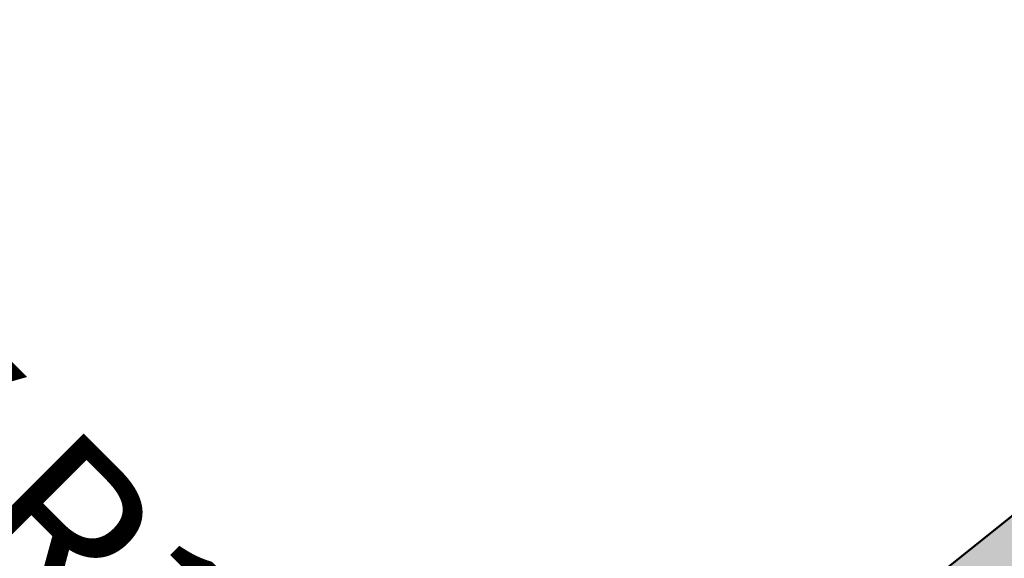
# Model space of a CAD drawing. Units: millimetres. Extents: x 0 to 2267, y 0 to 1823.
# Tile 19 of 256: x 1506 to 1548, y 1139 to 1162. Entities that reach past the tile are written whole.
import ezdxf

# ---------------------------------------------------------------- set-up
doc = ezdxf.new("R2010")
doc.units = ezdxf.units.MM
doc.header["$MEASUREMENT"] = 0
for name, color, linetype, lineweight in [('M-DIMS', 2, 'Continuous', 25), ('M-HATC', 252, 'Continuous', 18), ('M-OUTL', 7, 'Continuous', 50)]:
    doc.layers.add(name, color=color, linetype=linetype, lineweight=lineweight)
doc.styles.get("Standard").update_dxf_attribs({"font": 'arial.ttf'})
doc.dimstyles.get("Standard").update_dxf_attribs({"dimtxt": 7, "dimasz": 4, "dimexe": 0.18, "dimexo": 0.0625, "dimgap": 0.09, "dimtad": 0, "dimdec": 0, "dimzin": 0, "dimdsep": 46, "dimtxsty": 'Standard', "dimcen": 0.09, "dimadec": 0, "dimazin": 0, "dimtfac": 1, "dimtdec": 0, "dimtofl": 0, "dimtmove": 0, "dimatfit": 3, "dimfxl": 1, "dimtolj": 1, "dimtzin": 0, "dimarcsym": 0})

# ---------------------------------------------------------------- blocks, each defined once
blk = doc.blocks.new('*D28')
at = {"layer": 'Defpoints', "color": 0, "transparency": 16777216}
for p in [(1523.858, 1124.488), (1530.929, 1117.417)]:
    blk.add_point(p, dxfattribs=at)
at = {"layer": 'M-DIMS', "color": 0, "lineweight": -2, "transparency": 16777216}
for p, q in [((1518.201, 1130.145), (1521.029, 1127.317)), ((1530.929, 1117.327), (1530.929, 1117.507)), ((1530.839, 1117.417), (1531.019, 1117.417))]:
    blk.add_line(p, q, dxfattribs=at)
at = {"layer": 'M-DIMS', "color": 0, "transparency": 16777216}
blk.add_solid([(1521.501, 1127.788), (1520.558, 1126.845), (1523.858, 1124.488)], dxfattribs=at)
at = {"layer": 'M-DIMS', "color": 0, "transparency": 16777216, "insert": (1504.949, 1143.397), "char_height": 7, "attachment_point": 5, "rotation": 314.9998}
blk.add_mtext('\\A1;27X R10', dxfattribs=at)

msp = doc.modelspace()

# ---------------------------------------------------------------- hatches: boundary and pattern name
at = {"layer": 'M-HATC'}
h = msp.add_hatch(color=256, dxfattribs=at)
h.dxf.hatch_style = 1
h.paths.add_polyline_path([(2055.771, 1603.062), (1381.087, 1603.062), (1381.087, 1598.062), (2055.771, 1598.062)])
h.paths.add_polyline_path([(2055.771, 1598.062), (1381.087, 1598.062), (1381.087, 1593.062), (2055.771, 1593.062)])
h.paths.add_polyline_path([(2051.307, 1536.761), (1385.55, 1536.761), (1385.55, 1526.761), (1387.55, 1526.761), (1388.537, 1525.053), (1385.332, 1521.233), (1385.332, 1521.223), (2050.254, 1522.749), (2048.321, 1525.053), (2049.307, 1526.761), (2051.307, 1526.761)])
edge = h.paths.add_edge_path()
edge.add_arc((1847.535, 1379.149), 135, 222.60306, 222.89085, ccw=False)
edge.add_line((1748.166, 1287.766), (1683.092, 1287.766))
edge.add_arc((1583.724, 1379.149), 135, 317.10915, 317.39694, ccw=False)
edge.add_arc((1678.969, 1290.671), 5, 222.8909, 317.1091, ccw=False)
edge.add_arc((1774.213, 1379.149), 135, 222.60306, 222.89085, ccw=False)
edge.add_line((1674.845, 1287.766), (1609.771, 1287.766))
edge.add_arc((1510.403, 1379.149), 135, 317.10915, 317.39694, ccw=False)
edge.add_arc((1605.647, 1290.671), 5, 222.8909, 317.1091, ccw=False)
edge.add_arc((1700.892, 1379.149), 135, 222.60306, 222.89085, ccw=False)
edge.add_line((1601.524, 1287.766), (1536.45, 1287.766))
edge.add_arc((1437.081, 1379.149), 135, 317.10915, 317.39694, ccw=False)
edge.add_arc((1532.326, 1290.671), 5, 222.8909, 317.1091, ccw=False)
edge.add_arc((1627.571, 1379.149), 135, 222.60306, 222.89085, ccw=False)
edge.add_line((1528.203, 1287.766), (1505.929, 1287.766))
edge.add_spline(control_points=[(1505.929, 1287.766), (1504.262, 1287.766), (1504.262, 1282.766), (1505.929, 1282.766)], knot_values=[0, 0, 0, 0, 5, 5, 5, 5], degree=3, periodic=0)
edge.add_line((1505.929, 1282.766), (1930.929, 1282.766))
edge.add_spline(control_points=[(1930.929, 1282.766), (1932.596, 1282.766), (1932.596, 1287.766), (1930.929, 1287.766)], knot_values=[0, 0, 0, 0, 5, 5, 5, 5], degree=3, periodic=0)
edge.add_line((1930.929, 1287.766), (1903.056, 1287.766))
edge.add_arc((1803.688, 1379.149), 135, 317.10915, 317.39694, ccw=False)
edge.add_arc((1898.932, 1290.671), 5, 222.8909, 317.1091, ccw=False)
edge.add_arc((1994.177, 1379.149), 135, 222.60306, 222.89085, ccw=False)
edge.add_line((1894.809, 1287.766), (1829.735, 1287.766))
edge.add_arc((1730.366, 1379.149), 135, 317.10915, 317.39694, ccw=False)
edge.add_arc((1825.611, 1290.671), 5, 222.8909, 317.1091, ccw=False)
edge.add_arc((1920.856, 1379.149), 135, 222.60306, 222.89085, ccw=False)
edge.add_line((1821.487, 1287.766), (1756.413, 1287.766))
edge.add_arc((1657.045, 1379.149), 135, 317.10915, 317.39694, ccw=False)
edge.add_arc((1752.29, 1290.671), 5, 222.8909, 317.1091, ccw=False)
edge = h.paths.add_edge_path()
edge.add_spline(control_points=[(1843.429, 1227.247), (1845.096, 1227.247), (1845.096, 1232.247), (1843.429, 1232.247)], knot_values=[0, 0, 0, 0, 5, 5, 5, 5], degree=3, periodic=0)
edge.add_line((1843.429, 1232.247), (1593.429, 1232.247))
edge.add_spline(control_points=[(1593.429, 1232.247), (1591.762, 1232.247), (1591.762, 1227.247), (1593.429, 1227.247)], knot_values=[0, 0, 0, 0, 5, 5, 5, 5], degree=3, periodic=0)
edge.add_line((1593.429, 1227.247), (1843.429, 1227.247))
h.paths.add_polyline_path([(1905.929, 1127.417), (1530.929, 1127.417, 0.414214), (1520.929, 1117.417), (1530.929, 1117.417), (1915.929, 1117.417, 0.414214)])
edge = h.paths.add_edge_path()
edge.add_arc((1397.086, 1498.408), 12.73, 90.7821, 190.8787, ccw=False)
edge.add_line((1396.912, 1511.136), (1428.01, 1511.349))
edge.add_line((1428.01, 1511.349), (1433.01, 1511.349))
edge.add_line((1433.01, 1511.349), (1434.439, 1511.349))
edge.add_arc((1419.474, 1498.08), 20, 41.561, 74.0821)
edge.add_line((1424.959, 1517.314), (1399.935, 1517.256))
edge.add_spline(control_points=[(1399.931, 1517.256), (1399.884, 1517.213), (1399.833, 1517.169), (1399.777, 1517.124)], knot_values=[11.567499, 11.567499, 11.567499, 11.567499, 11.814249, 11.814249, 11.814249, 11.814249], degree=3, periodic=0)
edge.add_spline(control_points=[(1399.633, 1517.01), (1399.583, 1516.972), (1399.531, 1516.934), (1399.476, 1516.895)], knot_values=[11.167718, 11.167718, 11.167718, 11.167718, 11.365188, 11.365188, 11.365188, 11.365188], degree=3, periodic=0)
edge.add_spline(control_points=[(1399.34, 1516.8), (1399.151, 1516.672), (1398.938, 1516.538), (1398.704, 1516.399)], knot_values=[10.376405, 10.376405, 10.376405, 10.376405, 11.00994, 11.00994, 11.00994, 11.00994], degree=3, periodic=0)
edge.add_spline(control_points=[(1398.657, 1516.372), (1398.579, 1516.326), (1398.498, 1516.28), (1398.415, 1516.233)], knot_values=[10.125175, 10.125175, 10.125175, 10.125175, 10.334406, 10.334406, 10.334406, 10.334406], degree=3, periodic=0)
edge.add_spline(control_points=[(1398.264, 1516.149), (1398.196, 1516.111), (1398.126, 1516.073), (1398.055, 1516.035)], knot_values=[9.832246, 9.832246, 9.832246, 9.832246, 9.999658, 9.999658, 9.999658, 9.999658], degree=3, periodic=0)
edge.add_spline(control_points=[(1397.999, 1516.005), (1397.731, 1515.862), (1397.446, 1515.717), (1397.147, 1515.571)], knot_values=[9.161808, 9.161808, 9.161808, 9.161808, 9.787769, 9.787769, 9.787769, 9.787769], degree=3, periodic=0)
edge.add_spline(control_points=[(1397.147, 1515.571), (1396.842, 1515.423), (1396.522, 1515.274), (1396.191, 1515.126)], knot_values=[8.524455, 8.524455, 8.524455, 8.524455, 9.161808, 9.161808, 9.161808, 9.161808], degree=3, periodic=0)
edge.add_spline(control_points=[(1396.078, 1515.076), (1395.985, 1515.035), (1395.892, 1514.994), (1395.798, 1514.953)], knot_values=[8.275193, 8.275193, 8.275193, 8.275193, 8.451726, 8.451726, 8.451726, 8.451726], degree=3, periodic=0)
edge.add_spline(control_points=[(1395.602, 1514.869), (1395.5, 1514.826), (1395.397, 1514.782), (1395.293, 1514.739)], knot_values=[7.962917, 7.962917, 7.962917, 7.962917, 8.152764, 8.152764, 8.152764, 8.152764], degree=3, periodic=0)
edge.add_spline(control_points=[(1395.212, 1514.706), (1394.828, 1514.547), (1394.435, 1514.393), (1394.036, 1514.244)], knot_values=[7.21254, 7.21254, 7.21254, 7.21254, 7.913148, 7.913148, 7.913148, 7.913148], degree=3, periodic=0)
edge.add_spline(control_points=[(1394.036, 1514.244), (1393.708, 1514.121), (1393.375, 1514.003), (1393.043, 1513.889)], knot_values=[6.633733, 6.633733, 6.633733, 6.633733, 7.21254, 7.21254, 7.21254, 7.21254], degree=3, periodic=0)
edge.add_spline(control_points=[(1392.821, 1513.815), (1392.72, 1513.781), (1392.618, 1513.748), (1392.517, 1513.715)], knot_values=[6.328796, 6.328796, 6.328796, 6.328796, 6.505493, 6.505493, 6.505493, 6.505493], degree=3, periodic=0)
edge.add_spline(control_points=[(1392.517, 1513.715), (1392.319, 1513.652), (1392.121, 1513.59), (1391.924, 1513.531)], knot_values=[5.984605, 5.984605, 5.984605, 5.984605, 6.328796, 6.328796, 6.328796, 6.328796], degree=3, periodic=0)
edge.add_spline(control_points=[(1391.792, 1513.491), (1391.312, 1513.35), (1390.838, 1513.224), (1390.378, 1513.117)], knot_values=[5.066697, 5.066697, 5.066697, 5.066697, 5.907055, 5.907055, 5.907055, 5.907055], degree=3, periodic=0)
edge.add_spline(control_points=[(1390.378, 1513.117), (1390.18, 1513.071), (1389.984, 1513.028), (1389.791, 1512.99)], knot_values=[4.70367, 4.70367, 4.70367, 4.70367, 5.066695, 5.066695, 5.066695, 5.066695], degree=3, periodic=0)
edge.add_spline(control_points=[(1389.422, 1512.92), (1389.246, 1512.889), (1389.073, 1512.862), (1388.904, 1512.838)], knot_values=[4.130571, 4.130571, 4.130571, 4.130571, 4.469816, 4.469816, 4.469816, 4.469816], degree=3, periodic=0)
edge.add_spline(control_points=[(1388.904, 1512.838), (1388.591, 1512.795), (1388.291, 1512.764), (1388.007, 1512.749)], knot_values=[3.504031, 3.504031, 3.504031, 3.504031, 4.130571, 4.130571, 4.130571, 4.130571], degree=3, periodic=0)
edge.add_spline(control_points=[(1387.936, 1512.746), (1387.854, 1512.742), (1387.773, 1512.74), (1387.694, 1512.739)], knot_values=[3.268866, 3.268866, 3.268866, 3.268866, 3.451164, 3.451164, 3.451164, 3.451164], degree=3, periodic=0)
edge.add_spline(control_points=[(1387.335, 1512.744), (1387.208, 1512.75), (1387.085, 1512.76), (1386.967, 1512.774)], knot_values=[2.670686, 2.670686, 2.670686, 2.670686, 2.984, 2.984, 2.984, 2.984], degree=3, periodic=0)
edge.add_spline(control_points=[(1386.833, 1512.792), (1386.821, 1512.794), (1386.809, 1512.796), (1386.797, 1512.798)], knot_values=[2.516981, 2.516981, 2.516981, 2.516981, 2.549528, 2.549528, 2.549528, 2.549528], degree=3, periodic=0)
edge.add_spline(control_points=[(1386.453, 1512.873), (1386.426, 1512.881), (1386.399, 1512.889), (1386.373, 1512.897)], knot_values=[2.095869, 2.095869, 2.095869, 2.095869, 2.17941, 2.17941, 2.17941, 2.17941], degree=3, periodic=0)
edge.add_spline(control_points=[(1386.069, 1513.019), (1386.063, 1513.022), (1386.058, 1513.025), (1386.052, 1513.028)], knot_values=[1.72453, 1.72453, 1.72453, 1.72453, 1.745933, 1.745933, 1.745933, 1.745933], degree=3, periodic=0)
edge.add_arc((1399.474, 1498.08), 20, 131.8243, 180)
edge.add_arc((1630.334, 1505.548), 250.971, 181.70518, 236.42798)
edge.add_arc((1605.34, 1483.304), 218.782, 238.66083, 243.34961)
edge.add_arc((1647.091, 1510.359), 262.899, 183.12984, 237.85344, ccw=False)
h.paths.add_polyline_path([(1406.537, 1391.964, 0.149382), (1491.551, 1296.442, -0.129517)], flags=17)
edge = h.paths.add_edge_path()
edge.add_arc((2037.384, 1498.08), 20, 0, 48.2659)
edge.add_spline(control_points=[(2050.697, 1513.005), (2050.651, 1512.985), (2050.603, 1512.966), (2050.554, 1512.948)], knot_values=[1.835652, 1.835652, 1.835652, 1.835652, 2.000781, 2.000781, 2.000781, 2.000781], degree=3, periodic=0)
edge.add_spline(control_points=[(2050.462, 1512.917), (2050.479, 1512.922), (2050.496, 1512.928), (2050.513, 1512.934)], knot_values=[2.045477, 2.045477, 2.045477, 2.045477, 2.101389, 2.101389, 2.101389, 2.101389], degree=3, periodic=0)
edge.add_spline(control_points=[(2050.129, 1512.834), (2050.198, 1512.847), (2050.266, 1512.862), (2050.331, 1512.879)], knot_values=[2.237629, 2.237629, 2.237629, 2.237629, 2.435841, 2.435841, 2.435841, 2.435841], degree=3, periodic=0)
edge.add_spline(control_points=[(2050.095, 1512.828), (2050.106, 1512.83), (2050.118, 1512.832), (2050.129, 1512.834)], knot_values=[2.435841, 2.435841, 2.435841, 2.435841, 2.468321, 2.468321, 2.468321, 2.468321], degree=3, periodic=0)
edge.add_spline(control_points=[(2049.784, 1512.785), (2049.855, 1512.792), (2049.924, 1512.801), (2049.992, 1512.811)], knot_values=[2.563852, 2.563852, 2.563852, 2.563852, 2.748541, 2.748541, 2.748541, 2.748541], degree=3, periodic=0)
edge.add_spline(control_points=[(2049.405, 1512.762), (2049.536, 1512.765), (2049.663, 1512.773), (2049.784, 1512.785)], knot_values=[2.748541, 2.748541, 2.748541, 2.748541, 3.064882, 3.064882, 3.064882, 3.064882], degree=3, periodic=0)
edge.add_spline(control_points=[(2049.17, 1512.76), (2049.234, 1512.759), (2049.297, 1512.759), (2049.358, 1512.761)], knot_values=[3.102309, 3.102309, 3.102309, 3.102309, 3.2503, 3.2503, 3.2503, 3.2503], degree=3, periodic=0)
edge.add_spline(control_points=[(2048.857, 1512.769), (2048.964, 1512.764), (2049.068, 1512.761), (2049.17, 1512.76)], knot_values=[3.2503, 3.2503, 3.2503, 3.2503, 3.486069, 3.486069, 3.486069, 3.486069], degree=3, periodic=0)
edge.add_spline(control_points=[(2048.692, 1512.779), (2048.373, 1512.801), (2048.035, 1512.841), (2047.682, 1512.897)], knot_values=[3.606429, 3.606429, 3.606429, 3.606429, 4.2989, 4.2989, 4.2989, 4.2989], degree=3, periodic=0)
edge.add_spline(control_points=[(2047.682, 1512.897), (2047.546, 1512.919), (2047.408, 1512.942), (2047.268, 1512.969)], knot_values=[4.2989, 4.2989, 4.2989, 4.2989, 4.565769, 4.565769, 4.565769, 4.565769], degree=3, periodic=0)
edge.add_spline(control_points=[(2047.268, 1512.969), (2047.145, 1512.991), (2047.021, 1513.016), (2046.895, 1513.042)], knot_values=[4.565769, 4.565769, 4.565769, 4.565769, 4.799971, 4.799971, 4.799971, 4.799971], degree=3, periodic=0)
edge.add_spline(control_points=[(2046.895, 1513.042), (2046.529, 1513.119), (2046.151, 1513.209), (2045.768, 1513.311)], knot_values=[4.799971, 4.799971, 4.799971, 4.799971, 5.483718, 5.483718, 5.483718, 5.483718], degree=3, periodic=0)
edge.add_spline(control_points=[(2045.768, 1513.311), (2045.372, 1513.415), (2044.97, 1513.532), (2044.566, 1513.659)], knot_values=[5.483718, 5.483718, 5.483718, 5.483718, 6.187866, 6.187866, 6.187866, 6.187866], degree=3, periodic=0)
edge.add_spline(control_points=[(2044.566, 1513.659), (2044.415, 1513.706), (2044.263, 1513.755), (2044.112, 1513.805)], knot_values=[6.187866, 6.187866, 6.187866, 6.187866, 6.451551, 6.451551, 6.451551, 6.451551], degree=3, periodic=0)
edge.add_spline(control_points=[(2044.112, 1513.805), (2043.997, 1513.843), (2043.882, 1513.881), (2043.767, 1513.92)], knot_values=[6.451551, 6.451551, 6.451551, 6.451551, 6.651434, 6.651434, 6.651434, 6.651434], degree=3, periodic=0)
edge.add_spline(control_points=[(2043.767, 1513.92), (2043.372, 1514.055), (2042.977, 1514.198), (2042.589, 1514.346)], knot_values=[6.651434, 6.651434, 6.651434, 6.651434, 7.338879, 7.338879, 7.338879, 7.338879], degree=3, periodic=0)
edge.add_spline(control_points=[(2042.589, 1514.346), (2042.164, 1514.507), (2041.746, 1514.675), (2041.341, 1514.846)], knot_values=[7.338879, 7.338879, 7.338879, 7.338879, 8.089209, 8.089209, 8.089209, 8.089209], degree=3, periodic=0)
edge.add_spline(control_points=[(2041.341, 1514.846), (2041.103, 1514.946), (2040.869, 1515.048), (2040.64, 1515.15)], knot_values=[8.089209, 8.089209, 8.089209, 8.089209, 8.529587, 8.529587, 8.529587, 8.529587], degree=3, periodic=0)
edge.add_spline(control_points=[(2040.51, 1515.209), (2040.082, 1515.402), (2039.675, 1515.597), (2039.295, 1515.789)], knot_values=[8.613818, 8.613818, 8.613818, 8.613818, 9.44571, 9.44571, 9.44571, 9.44571], degree=3, periodic=0)
edge.add_spline(control_points=[(2039.295, 1515.789), (2039.062, 1515.907), (2038.839, 1516.025), (2038.629, 1516.14)], knot_values=[9.44571, 9.44571, 9.44571, 9.44571, 9.956404, 9.956404, 9.956404, 9.956404], degree=3, periodic=0)
edge.add_spline(control_points=[(2038.629, 1516.14), (2038.519, 1516.2), (2038.412, 1516.26), (2038.309, 1516.319)], knot_values=[9.956404, 9.956404, 9.956404, 9.956404, 10.223542, 10.223542, 10.223542, 10.223542], degree=3, periodic=0)
edge.add_spline(control_points=[(2038.309, 1516.319), (2038.214, 1516.374), (2038.122, 1516.428), (2038.033, 1516.481)], knot_values=[10.223542, 10.223542, 10.223542, 10.223542, 10.47051, 10.47051, 10.47051, 10.47051], degree=3, periodic=0)
edge.add_spline(control_points=[(2038.033, 1516.481), (2037.786, 1516.63), (2037.564, 1516.773), (2037.372, 1516.909)], knot_values=[10.47051, 10.47051, 10.47051, 10.47051, 11.15767, 11.15767, 11.15767, 11.15767], degree=3, periodic=0)
edge.add_spline(control_points=[(2037.372, 1516.909), (2037.279, 1516.975), (2037.193, 1517.04), (2037.114, 1517.102)], knot_values=[11.15767, 11.15767, 11.15767, 11.15767, 11.49227, 11.49227, 11.49227, 11.49227], degree=3, periodic=0)
edge.add_spline(control_points=[(2036.856, 1517.326), (2036.915, 1517.269), (2036.981, 1517.21), (2037.056, 1517.149)], knot_values=[11.577341, 11.577341, 11.577341, 11.577341, 11.91035, 11.91035, 11.91035, 11.91035], degree=3, periodic=0)
edge.add_spline(control_points=[(2036.807, 1517.375), (2036.823, 1517.359), (2036.839, 1517.342), (2036.856, 1517.326)], knot_values=[11.91035, 11.91035, 11.91035, 11.91035, 12.007402, 12.007402, 12.007402, 12.007402], degree=3, periodic=0)
edge.add_spline(control_points=[(2036.702, 1517.494), (2036.71, 1517.483), (2036.72, 1517.472), (2036.729, 1517.461)], knot_values=[12.184155, 12.184155, 12.184155, 12.184155, 12.255409, 12.255409, 12.255409, 12.255409], degree=3, periodic=0)
edge.add_spline(control_points=[(2036.616, 1517.621), (2036.62, 1517.613), (2036.624, 1517.606), (2036.629, 1517.598)], knot_values=[12.487913, 12.487913, 12.487913, 12.487913, 12.541035, 12.541035, 12.541035, 12.541035], degree=3, periodic=0)
edge.add_spline(control_points=[(2036.563, 1517.786), (2036.564, 1517.779), (2036.564, 1517.773), (2036.565, 1517.766)], knot_values=[12.911761, 12.911761, 12.911761, 12.911761, 12.968286, 12.968286, 12.968286, 12.968286], degree=3, periodic=0)
edge.add_spline(control_points=[(2036.617, 1517.93), (2036.612, 1517.926), (2036.609, 1517.921), (2036.605, 1517.916)], knot_values=[13.382527, 13.382527, 13.382527, 13.382527, 13.433791, 13.433791, 13.433791, 13.433791], degree=3, periodic=0)
edge.add_spline(control_points=[(2036.749, 1518.017), (2036.736, 1518.012), (2036.724, 1518.006), (2036.712, 1518)], knot_values=[13.726299, 13.726299, 13.726299, 13.726299, 13.809928, 13.809928, 13.809928, 13.809928], degree=3, periodic=0)
edge.add_spline(control_points=[(2036.86, 1518.053), (2036.839, 1518.047), (2036.818, 1518.042), (2036.799, 1518.035)], knot_values=[13.910887, 13.910887, 13.910887, 13.910887, 14.02153, 14.02153, 14.02153, 14.02153], degree=3, periodic=0)
edge.add_line((2036.964, 1518.08), (2032.384, 1518.08))
edge.add_line((2032.384, 1518.08), (2027.384, 1518.08))
edge.add_line((2027.384, 1518.08), (2022.384, 1518.08))
edge.add_line((2022.384, 1518.08), (2017.384, 1518.08))
edge.add_arc((2017.384, 1498.08), 20, 90, 138.439)
edge.add_line((2002.419, 1511.349), (2003.848, 1511.349))
edge.add_line((2003.848, 1511.349), (2008.848, 1511.349))
edge.add_line((2008.848, 1511.349), (2039.772, 1511.138))
edge.add_arc((2039.772, 1498.408), 12.73, -10.8787, 90, ccw=False)
edge.add_arc((1789.767, 1510.359), 262.899, 302.14656, 356.87016, ccw=False)
edge.add_arc((1831.518, 1483.304), 218.782, 296.65039, 301.33917)
edge.add_arc((1806.524, 1505.548), 250.971, 303.57202, 358.29482)
h.paths.add_polyline_path([(2030.321, 1391.964, -0.129517), (1945.307, 1296.442, 0.149382)], flags=17)
edge = h.paths.add_edge_path()
edge.add_spline(control_points=[(2037.246, 1518.082), (2037.29, 1518.081), (2037.336, 1518.08), (2037.384, 1518.08)], knot_values=[0.000012, 0.000012, 0.000012, 0.000012, 0.144754, 0.144754, 0.144754, 0.144754], degree=3, periodic=0)
edge.add_line((2037.336, 1518.08), (2037.01, 1518.08))
edge.add_spline(control_points=[(2037.01, 1518.08), (2036.982, 1518.077), (2036.956, 1518.073), (2036.931, 1518.068)], knot_values=[14.13465, 14.13465, 14.13465, 14.13465, 14.247197, 14.247197, 14.247197, 14.247197], degree=3, periodic=0)
edge.add_spline(control_points=[(2036.931, 1518.068), (2036.928, 1518.067), (2036.924, 1518.067), (2036.921, 1518.066)], knot_values=[14.118315, 14.118315, 14.118315, 14.118315, 14.13465, 14.13465, 14.13465, 14.13465], degree=3, periodic=0)
edge.add_spline(control_points=[(2036.921, 1518.066), (2036.912, 1518.064), (2036.903, 1518.063), (2036.895, 1518.061)], knot_values=[14.078086, 14.078086, 14.078086, 14.078086, 14.118315, 14.118315, 14.118315, 14.118315], degree=3, periodic=0)
edge.add_spline(control_points=[(2036.895, 1518.061), (2036.883, 1518.058), (2036.872, 1518.056), (2036.86, 1518.053)], knot_values=[14.02153, 14.02153, 14.02153, 14.02153, 14.078086, 14.078086, 14.078086, 14.078086], degree=3, periodic=0)
edge.add_spline(control_points=[(2036.86, 1518.053), (2036.839, 1518.047), (2036.818, 1518.042), (2036.799, 1518.035)], knot_values=[13.910887, 13.910887, 13.910887, 13.910887, 14.02153, 14.02153, 14.02153, 14.02153], degree=3, periodic=0)
edge.add_spline(control_points=[(2036.799, 1518.035), (2036.798, 1518.035), (2036.797, 1518.035), (2036.797, 1518.035)], knot_values=[13.906906, 13.906906, 13.906906, 13.906906, 13.910887, 13.910887, 13.910887, 13.910887], degree=3, periodic=0)
edge.add_spline(control_points=[(2036.797, 1518.035), (2036.788, 1518.032), (2036.78, 1518.029), (2036.772, 1518.026)], knot_values=[13.857826, 13.857826, 13.857826, 13.857826, 13.906906, 13.906906, 13.906906, 13.906906], degree=3, periodic=0)
edge.add_spline(control_points=[(2036.772, 1518.026), (2036.764, 1518.023), (2036.756, 1518.02), (2036.749, 1518.017)], knot_values=[13.809928, 13.809928, 13.809928, 13.809928, 13.857826, 13.857826, 13.857826, 13.857826], degree=3, periodic=0)
edge.add_spline(control_points=[(2036.749, 1518.017), (2036.736, 1518.012), (2036.724, 1518.006), (2036.712, 1518)], knot_values=[13.726299, 13.726299, 13.726299, 13.726299, 13.809928, 13.809928, 13.809928, 13.809928], degree=3, periodic=0)
edge.add_spline(control_points=[(2036.712, 1518), (2036.712, 1518), (2036.712, 1518), (2036.711, 1518)], knot_values=[13.723993, 13.723993, 13.723993, 13.723993, 13.726299, 13.726299, 13.726299, 13.726299], degree=3, periodic=0)
edge.add_spline(control_points=[(2036.711, 1518), (2036.706, 1517.997), (2036.701, 1517.994), (2036.696, 1517.992)], knot_values=[13.686536, 13.686536, 13.686536, 13.686536, 13.723993, 13.723993, 13.723993, 13.723993], degree=3, periodic=0)
edge.add_spline(control_points=[(2036.696, 1517.992), (2036.692, 1517.989), (2036.687, 1517.987), (2036.683, 1517.984)], knot_values=[13.651251, 13.651251, 13.651251, 13.651251, 13.686536, 13.686536, 13.686536, 13.686536], degree=3, periodic=0)
edge.add_spline(control_points=[(2036.683, 1517.984), (2036.676, 1517.98), (2036.67, 1517.976), (2036.664, 1517.971)], knot_values=[13.596804, 13.596804, 13.596804, 13.596804, 13.651251, 13.651251, 13.651251, 13.651251], degree=3, periodic=0)
edge.add_spline(control_points=[(2036.664, 1517.971), (2036.664, 1517.971), (2036.663, 1517.971), (2036.663, 1517.971)], knot_values=[13.593956, 13.593956, 13.593956, 13.593956, 13.596804, 13.596804, 13.596804, 13.596804], degree=3, periodic=0)
edge.add_spline(control_points=[(2036.663, 1517.971), (2036.66, 1517.969), (2036.658, 1517.967), (2036.655, 1517.965)], knot_values=[13.570322, 13.570322, 13.570322, 13.570322, 13.593956, 13.593956, 13.593956, 13.593956], degree=3, periodic=0)
edge.add_spline(control_points=[(2036.655, 1517.965), (2036.653, 1517.963), (2036.65, 1517.961), (2036.647, 1517.959)], knot_values=[13.545477, 13.545477, 13.545477, 13.545477, 13.570322, 13.570322, 13.570322, 13.570322], degree=3, periodic=0)
edge.add_spline(control_points=[(2036.647, 1517.959), (2036.647, 1517.959), (2036.647, 1517.959), (2036.647, 1517.959)], knot_values=[13.543931, 13.543931, 13.543931, 13.543931, 13.545477, 13.545477, 13.545477, 13.545477], degree=3, periodic=0)
edge.add_spline(control_points=[(2036.647, 1517.959), (2036.641, 1517.954), (2036.636, 1517.949), (2036.631, 1517.945)], knot_values=[13.488237, 13.488237, 13.488237, 13.488237, 13.543931, 13.543931, 13.543931, 13.543931], degree=3, periodic=0)
edge.add_spline(control_points=[(2036.631, 1517.945), (2036.628, 1517.942), (2036.626, 1517.94), (2036.623, 1517.937)], knot_values=[13.460307, 13.460307, 13.460307, 13.460307, 13.488237, 13.488237, 13.488237, 13.488237], degree=3, periodic=0)
edge.add_spline(control_points=[(2036.623, 1517.937), (2036.622, 1517.936), (2036.62, 1517.934), (2036.618, 1517.932)], knot_values=[13.439712, 13.439712, 13.439712, 13.439712, 13.460307, 13.460307, 13.460307, 13.460307], degree=3, periodic=0)
edge.add_spline(control_points=[(2036.618, 1517.932), (2036.618, 1517.931), (2036.617, 1517.931), (2036.617, 1517.93)], knot_values=[13.433791, 13.433791, 13.433791, 13.433791, 13.439712, 13.439712, 13.439712, 13.439712], degree=3, periodic=0)
edge.add_spline(control_points=[(2036.617, 1517.93), (2036.612, 1517.926), (2036.609, 1517.921), (2036.605, 1517.916)], knot_values=[13.382527, 13.382527, 13.382527, 13.382527, 13.433791, 13.433791, 13.433791, 13.433791], degree=3, periodic=0)
edge.add_spline(control_points=[(2036.605, 1517.916), (2036.603, 1517.913), (2036.6, 1517.91), (2036.598, 1517.907)], knot_values=[13.350017, 13.350017, 13.350017, 13.350017, 13.382527, 13.382527, 13.382527, 13.382527], degree=3, periodic=0)
edge.add_spline(control_points=[(2036.598, 1517.907), (2036.597, 1517.906), (2036.596, 1517.904), (2036.595, 1517.903)], knot_values=[13.333922, 13.333922, 13.333922, 13.333922, 13.350017, 13.350017, 13.350017, 13.350017], degree=3, periodic=0)
edge.add_spline(control_points=[(2036.595, 1517.903), (2036.595, 1517.902), (2036.594, 1517.901), (2036.593, 1517.9)], knot_values=[13.323828, 13.323828, 13.323828, 13.323828, 13.333922, 13.333922, 13.333922, 13.333922], degree=3, periodic=0)
edge.add_spline(control_points=[(2036.593, 1517.9), (2036.59, 1517.895), (2036.588, 1517.891), (2036.585, 1517.886)], knot_values=[13.277545, 13.277545, 13.277545, 13.277545, 13.323828, 13.323828, 13.323828, 13.323828], degree=3, periodic=0)
edge.add_spline(control_points=[(2036.585, 1517.886), (2036.584, 1517.883), (2036.582, 1517.879), (2036.58, 1517.875)], knot_values=[13.240119, 13.240119, 13.240119, 13.240119, 13.277545, 13.277545, 13.277545, 13.277545], degree=3, periodic=0)
edge.add_spline(control_points=[(2036.58, 1517.875), (2036.58, 1517.874), (2036.579, 1517.873), (2036.578, 1517.872)], knot_values=[13.228211, 13.228211, 13.228211, 13.228211, 13.240119, 13.240119, 13.240119, 13.240119], degree=3, periodic=0)
edge.add_spline(control_points=[(2036.578, 1517.872), (2036.578, 1517.87), (2036.577, 1517.869), (2036.577, 1517.868)], knot_values=[13.215717, 13.215717, 13.215717, 13.215717, 13.228211, 13.228211, 13.228211, 13.228211], degree=3, periodic=0)
edge.add_spline(control_points=[(2036.577, 1517.868), (2036.575, 1517.864), (2036.574, 1517.86), (2036.573, 1517.857)], knot_values=[13.179847, 13.179847, 13.179847, 13.179847, 13.215717, 13.215717, 13.215717, 13.215717], degree=3, periodic=0)
edge.add_spline(control_points=[(2036.573, 1517.857), (2036.571, 1517.851), (2036.57, 1517.846), (2036.569, 1517.841)], knot_values=[13.132017, 13.132017, 13.132017, 13.132017, 13.179847, 13.179847, 13.179847, 13.179847], degree=3, periodic=0)
edge.add_spline(control_points=[(2036.569, 1517.841), (2036.568, 1517.84), (2036.568, 1517.839), (2036.568, 1517.838)], knot_values=[13.122482, 13.122482, 13.122482, 13.122482, 13.132017, 13.132017, 13.132017, 13.132017], degree=3, periodic=0)
edge.add_spline(control_points=[(2036.568, 1517.838), (2036.568, 1517.836), (2036.567, 1517.835), (2036.567, 1517.833)], knot_values=[13.105592, 13.105592, 13.105592, 13.105592, 13.122482, 13.122482, 13.122482, 13.122482], degree=3, periodic=0)
edge.add_spline(control_points=[(2036.567, 1517.833), (2036.566, 1517.829), (2036.566, 1517.826), (2036.565, 1517.822)], knot_values=[13.074063, 13.074063, 13.074063, 13.074063, 13.105592, 13.105592, 13.105592, 13.105592], degree=3, periodic=0)
edge.add_spline(control_points=[(2036.565, 1517.822), (2036.565, 1517.822), (2036.565, 1517.822), (2036.565, 1517.822)], knot_values=[13.074043, 13.074043, 13.074043, 13.074043, 13.074063, 13.074063, 13.074063, 13.074063], degree=3, periodic=0)
edge.add_spline(control_points=[(2036.565, 1517.822), (2036.564, 1517.816), (2036.564, 1517.811), (2036.564, 1517.805)], knot_values=[13.021884, 13.021884, 13.021884, 13.021884, 13.074043, 13.074043, 13.074043, 13.074043], degree=3, periodic=0)
edge.add_spline(control_points=[(2036.564, 1517.805), (2036.564, 1517.804), (2036.564, 1517.803), (2036.564, 1517.803)], knot_values=[13.01674, 13.01674, 13.01674, 13.01674, 13.021884, 13.021884, 13.021884, 13.021884], degree=3, periodic=0)
edge.add_spline(control_points=[(2036.564, 1517.803), (2036.563, 1517.801), (2036.563, 1517.798), (2036.563, 1517.796)], knot_values=[12.996438, 12.996438, 12.996438, 12.996438, 13.01674, 13.01674, 13.01674, 13.01674], degree=3, periodic=0)
edge.add_spline(control_points=[(2036.563, 1517.796), (2036.563, 1517.793), (2036.563, 1517.789), (2036.563, 1517.786)], knot_values=[12.968286, 12.968286, 12.968286, 12.968286, 12.996438, 12.996438, 12.996438, 12.996438], degree=3, periodic=0)
edge.add_spline(control_points=[(2036.563, 1517.786), (2036.564, 1517.779), (2036.564, 1517.773), (2036.565, 1517.766)], knot_values=[12.911761, 12.911761, 12.911761, 12.911761, 12.968286, 12.968286, 12.968286, 12.968286], degree=3, periodic=0)
edge.add_spline(control_points=[(2036.565, 1517.766), (2036.565, 1517.766), (2036.565, 1517.766), (2036.565, 1517.766)], knot_values=[12.911017, 12.911017, 12.911017, 12.911017, 12.911761, 12.911761, 12.911761, 12.911761], degree=3, periodic=0)
edge.add_spline(control_points=[(2036.565, 1517.766), (2036.565, 1517.762), (2036.566, 1517.759), (2036.566, 1517.756)], knot_values=[12.88528, 12.88528, 12.88528, 12.88528, 12.911017, 12.911017, 12.911017, 12.911017], degree=3, periodic=0)
edge.add_spline(control_points=[(2036.566, 1517.756), (2036.567, 1517.753), (2036.567, 1517.751), (2036.568, 1517.748)], knot_values=[12.862519, 12.862519, 12.862519, 12.862519, 12.88528, 12.88528, 12.88528, 12.88528], degree=3, periodic=0)
edge.add_spline(control_points=[(2036.568, 1517.748), (2036.568, 1517.747), (2036.568, 1517.747), (2036.568, 1517.746)], knot_values=[12.858885, 12.858885, 12.858885, 12.858885, 12.862519, 12.862519, 12.862519, 12.862519], degree=3, periodic=0)
edge.add_spline(control_points=[(2036.568, 1517.746), (2036.569, 1517.74), (2036.571, 1517.733), (2036.572, 1517.726)], knot_values=[12.8053, 12.8053, 12.8053, 12.8053, 12.858885, 12.858885, 12.858885, 12.858885], degree=3, periodic=0)
edge.add_spline(control_points=[(2036.572, 1517.726), (2036.573, 1517.723), (2036.574, 1517.719), (2036.576, 1517.715)], knot_values=[12.775176, 12.775176, 12.775176, 12.775176, 12.8053, 12.8053, 12.8053, 12.8053], degree=3, periodic=0)
edge.add_spline(control_points=[(2036.576, 1517.715), (2036.576, 1517.713), (2036.577, 1517.71), (2036.578, 1517.708)], knot_values=[12.756759, 12.756759, 12.756759, 12.756759, 12.775176, 12.775176, 12.775176, 12.775176], degree=3, periodic=0)
edge.add_spline(control_points=[(2036.578, 1517.708), (2036.578, 1517.707), (2036.578, 1517.706), (2036.579, 1517.705)], knot_values=[12.748742, 12.748742, 12.748742, 12.748742, 12.756759, 12.756759, 12.756759, 12.756759], degree=3, periodic=0)
edge.add_spline(control_points=[(2036.579, 1517.705), (2036.581, 1517.698), (2036.583, 1517.692), (2036.586, 1517.685)], knot_values=[12.69959, 12.69959, 12.69959, 12.69959, 12.748742, 12.748742, 12.748742, 12.748742], degree=3, periodic=0)
edge.add_spline(control_points=[(2036.586, 1517.685), (2036.588, 1517.68), (2036.59, 1517.675), (2036.592, 1517.669)], knot_values=[12.659038, 12.659038, 12.659038, 12.659038, 12.69959, 12.69959, 12.69959, 12.69959], degree=3, periodic=0)
edge.add_spline(control_points=[(2036.592, 1517.669), (2036.594, 1517.665), (2036.596, 1517.66), (2036.598, 1517.656)], knot_values=[12.626806, 12.626806, 12.626806, 12.626806, 12.659038, 12.659038, 12.659038, 12.659038], degree=3, periodic=0)
edge.add_spline(control_points=[(2036.598, 1517.656), (2036.598, 1517.655), (2036.599, 1517.654), (2036.599, 1517.653)], knot_values=[12.619394, 12.619394, 12.619394, 12.619394, 12.626806, 12.626806, 12.626806, 12.626806], degree=3, periodic=0)
edge.add_spline(control_points=[(2036.599, 1517.653), (2036.604, 1517.642), (2036.61, 1517.632), (2036.616, 1517.621)], knot_values=[12.541039, 12.541039, 12.541039, 12.541039, 12.619394, 12.619394, 12.619394, 12.619394], degree=3, periodic=0)
edge.add_spline(control_points=[(2036.616, 1517.621), (2036.616, 1517.621), (2036.616, 1517.621), (2036.616, 1517.621)], knot_values=[12.541035, 12.541035, 12.541035, 12.541035, 12.541039, 12.541039, 12.541039, 12.541039], degree=3, periodic=0)
edge.add_spline(control_points=[(2036.616, 1517.621), (2036.62, 1517.613), (2036.624, 1517.606), (2036.629, 1517.598)], knot_values=[12.487913, 12.487913, 12.487913, 12.487913, 12.541035, 12.541035, 12.541035, 12.541035], degree=3, periodic=0)
edge.add_spline(control_points=[(2036.629, 1517.598), (2036.633, 1517.592), (2036.637, 1517.585), (2036.641, 1517.579)], knot_values=[12.443982, 12.443982, 12.443982, 12.443982, 12.487913, 12.487913, 12.487913, 12.487913], degree=3, periodic=0)
edge.add_spline(control_points=[(2036.641, 1517.579), (2036.641, 1517.578), (2036.642, 1517.576), (2036.643, 1517.575)], knot_values=[12.434996, 12.434996, 12.434996, 12.434996, 12.443982, 12.443982, 12.443982, 12.443982], degree=3, periodic=0)
edge.add_spline(control_points=[(2036.643, 1517.575), (2036.653, 1517.56), (2036.664, 1517.544), (2036.676, 1517.528)], knot_values=[12.329647, 12.329647, 12.329647, 12.329647, 12.434996, 12.434996, 12.434996, 12.434996], degree=3, periodic=0)
edge.add_spline(control_points=[(2036.676, 1517.528), (2036.684, 1517.517), (2036.693, 1517.505), (2036.702, 1517.494)], knot_values=[12.255409, 12.255409, 12.255409, 12.255409, 12.329647, 12.329647, 12.329647, 12.329647], degree=3, periodic=0)
edge.add_spline(control_points=[(2036.702, 1517.494), (2036.71, 1517.483), (2036.72, 1517.472), (2036.729, 1517.461)], knot_values=[12.184155, 12.184155, 12.184155, 12.184155, 12.255409, 12.255409, 12.255409, 12.255409], degree=3, periodic=0)
edge.add_spline(control_points=[(2036.729, 1517.461), (2036.744, 1517.444), (2036.759, 1517.426), (2036.775, 1517.409)], knot_values=[12.075961, 12.075961, 12.075961, 12.075961, 12.184155, 12.184155, 12.184155, 12.184155], degree=3, periodic=0)
edge.add_spline(control_points=[(2036.775, 1517.409), (2036.776, 1517.407), (2036.777, 1517.406), (2036.778, 1517.405)], knot_values=[12.069502, 12.069502, 12.069502, 12.069502, 12.075961, 12.075961, 12.075961, 12.075961], degree=3, periodic=0)
edge.add_spline(control_points=[(2036.778, 1517.405), (2036.788, 1517.395), (2036.797, 1517.385), (2036.807, 1517.375)], knot_values=[12.007402, 12.007402, 12.007402, 12.007402, 12.069502, 12.069502, 12.069502, 12.069502], degree=3, periodic=0)
edge.add_spline(control_points=[(2036.807, 1517.375), (2036.823, 1517.359), (2036.839, 1517.342), (2036.856, 1517.326)], knot_values=[11.91035, 11.91035, 11.91035, 11.91035, 12.007402, 12.007402, 12.007402, 12.007402], degree=3, periodic=0)
edge.add_spline(control_points=[(2036.856, 1517.326), (2036.915, 1517.269), (2036.981, 1517.21), (2037.056, 1517.149)], knot_values=[11.577341, 11.577341, 11.577341, 11.577341, 11.91035, 11.91035, 11.91035, 11.91035], degree=3, periodic=0)
edge.add_spline(control_points=[(2037.056, 1517.149), (2037.075, 1517.134), (2037.094, 1517.118), (2037.114, 1517.102)], knot_values=[11.49227, 11.49227, 11.49227, 11.49227, 11.577341, 11.577341, 11.577341, 11.577341], degree=3, periodic=0)
edge.add_spline(control_points=[(2037.114, 1517.102), (2037.193, 1517.04), (2037.279, 1516.975), (2037.372, 1516.909)], knot_values=[11.15767, 11.15767, 11.15767, 11.15767, 11.49227, 11.49227, 11.49227, 11.49227], degree=3, periodic=0)
edge.add_spline(control_points=[(2037.372, 1516.909), (2037.564, 1516.773), (2037.786, 1516.63), (2038.033, 1516.481)], knot_values=[10.47051, 10.47051, 10.47051, 10.47051, 11.15767, 11.15767, 11.15767, 11.15767], degree=3, periodic=0)
edge.add_spline(control_points=[(2038.033, 1516.481), (2038.122, 1516.428), (2038.214, 1516.374), (2038.309, 1516.319)], knot_values=[10.223542, 10.223542, 10.223542, 10.223542, 10.47051, 10.47051, 10.47051, 10.47051], degree=3, periodic=0)
edge.add_spline(control_points=[(2038.309, 1516.319), (2038.412, 1516.26), (2038.519, 1516.2), (2038.629, 1516.14)], knot_values=[9.956404, 9.956404, 9.956404, 9.956404, 10.223542, 10.223542, 10.223542, 10.223542], degree=3, periodic=0)
edge.add_spline(control_points=[(2038.629, 1516.14), (2038.839, 1516.025), (2039.062, 1515.907), (2039.295, 1515.789)], knot_values=[9.44571, 9.44571, 9.44571, 9.44571, 9.956404, 9.956404, 9.956404, 9.956404], degree=3, periodic=0)
edge.add_spline(control_points=[(2039.295, 1515.789), (2039.675, 1515.597), (2040.082, 1515.402), (2040.51, 1515.209)], knot_values=[8.613818, 8.613818, 8.613818, 8.613818, 9.44571, 9.44571, 9.44571, 9.44571], degree=3, periodic=0)
edge.add_spline(control_points=[(2040.51, 1515.209), (2040.553, 1515.189), (2040.597, 1515.17), (2040.64, 1515.15)], knot_values=[8.529587, 8.529587, 8.529587, 8.529587, 8.613818, 8.613818, 8.613818, 8.613818], degree=3, periodic=0)
edge.add_spline(control_points=[(2040.64, 1515.15), (2040.869, 1515.048), (2041.103, 1514.946), (2041.341, 1514.846)], knot_values=[8.089209, 8.089209, 8.089209, 8.089209, 8.529587, 8.529587, 8.529587, 8.529587], degree=3, periodic=0)
edge.add_spline(control_points=[(2041.341, 1514.846), (2041.746, 1514.675), (2042.164, 1514.507), (2042.589, 1514.346)], knot_values=[7.338879, 7.338879, 7.338879, 7.338879, 8.089209, 8.089209, 8.089209, 8.089209], degree=3, periodic=0)
edge.add_spline(control_points=[(2042.589, 1514.346), (2042.977, 1514.198), (2043.372, 1514.055), (2043.767, 1513.92)], knot_values=[6.651434, 6.651434, 6.651434, 6.651434, 7.338879, 7.338879, 7.338879, 7.338879], degree=3, periodic=0)
edge.add_spline(control_points=[(2043.767, 1513.92), (2043.882, 1513.881), (2043.997, 1513.843), (2044.112, 1513.805)], knot_values=[6.451551, 6.451551, 6.451551, 6.451551, 6.651434, 6.651434, 6.651434, 6.651434], degree=3, periodic=0)
edge.add_spline(control_points=[(2044.112, 1513.805), (2044.263, 1513.755), (2044.415, 1513.706), (2044.566, 1513.659)], knot_values=[6.187866, 6.187866, 6.187866, 6.187866, 6.451551, 6.451551, 6.451551, 6.451551], degree=3, periodic=0)
edge.add_spline(control_points=[(2044.566, 1513.659), (2044.97, 1513.532), (2045.372, 1513.415), (2045.768, 1513.311)], knot_values=[5.483718, 5.483718, 5.483718, 5.483718, 6.187866, 6.187866, 6.187866, 6.187866], degree=3, periodic=0)
edge.add_spline(control_points=[(2045.768, 1513.311), (2046.151, 1513.209), (2046.529, 1513.119), (2046.895, 1513.042)], knot_values=[4.799971, 4.799971, 4.799971, 4.799971, 5.483718, 5.483718, 5.483718, 5.483718], degree=3, periodic=0)
edge.add_spline(control_points=[(2046.895, 1513.042), (2047.021, 1513.016), (2047.145, 1512.991), (2047.268, 1512.969)], knot_values=[4.565769, 4.565769, 4.565769, 4.565769, 4.799971, 4.799971, 4.799971, 4.799971], degree=3, periodic=0)
edge.add_spline(control_points=[(2047.268, 1512.969), (2047.408, 1512.942), (2047.546, 1512.919), (2047.682, 1512.897)], knot_values=[4.2989, 4.2989, 4.2989, 4.2989, 4.565769, 4.565769, 4.565769, 4.565769], degree=3, periodic=0)
edge.add_spline(control_points=[(2047.682, 1512.897), (2048.035, 1512.841), (2048.373, 1512.801), (2048.692, 1512.779)], knot_values=[3.606429, 3.606429, 3.606429, 3.606429, 4.2989, 4.2989, 4.2989, 4.2989], degree=3, periodic=0)
edge.add_spline(control_points=[(2048.692, 1512.779), (2048.748, 1512.775), (2048.803, 1512.772), (2048.857, 1512.769)], knot_values=[3.486069, 3.486069, 3.486069, 3.486069, 3.606429, 3.606429, 3.606429, 3.606429], degree=3, periodic=0)
edge.add_spline(control_points=[(2048.857, 1512.769), (2048.964, 1512.764), (2049.068, 1512.761), (2049.17, 1512.76)], knot_values=[3.2503, 3.2503, 3.2503, 3.2503, 3.486069, 3.486069, 3.486069, 3.486069], degree=3, periodic=0)
edge.add_spline(control_points=[(2049.17, 1512.76), (2049.234, 1512.759), (2049.297, 1512.759), (2049.358, 1512.761)], knot_values=[3.102309, 3.102309, 3.102309, 3.102309, 3.2503, 3.2503, 3.2503, 3.2503], degree=3, periodic=0)
edge.add_spline(control_points=[(2049.358, 1512.761), (2049.374, 1512.761), (2049.39, 1512.761), (2049.405, 1512.762)], knot_values=[3.064882, 3.064882, 3.064882, 3.064882, 3.102309, 3.102309, 3.102309, 3.102309], degree=3, periodic=0)
edge.add_spline(control_points=[(2049.405, 1512.762), (2049.536, 1512.765), (2049.663, 1512.773), (2049.784, 1512.785)], knot_values=[2.748541, 2.748541, 2.748541, 2.748541, 3.064882, 3.064882, 3.064882, 3.064882], degree=3, periodic=0)
edge.add_spline(control_points=[(2049.784, 1512.785), (2049.855, 1512.792), (2049.924, 1512.801), (2049.992, 1512.811)], knot_values=[2.563852, 2.563852, 2.563852, 2.563852, 2.748541, 2.748541, 2.748541, 2.748541], degree=3, periodic=0)
edge.add_spline(control_points=[(2049.992, 1512.811), (2050.026, 1512.816), (2050.061, 1512.822), (2050.095, 1512.828)], knot_values=[2.468321, 2.468321, 2.468321, 2.468321, 2.563852, 2.563852, 2.563852, 2.563852], degree=3, periodic=0)
edge.add_spline(control_points=[(2050.095, 1512.828), (2050.106, 1512.83), (2050.118, 1512.832), (2050.129, 1512.834)], knot_values=[2.435841, 2.435841, 2.435841, 2.435841, 2.468321, 2.468321, 2.468321, 2.468321], degree=3, periodic=0)
edge.add_spline(control_points=[(2050.129, 1512.834), (2050.198, 1512.847), (2050.266, 1512.862), (2050.331, 1512.879)], knot_values=[2.237629, 2.237629, 2.237629, 2.237629, 2.435841, 2.435841, 2.435841, 2.435841], degree=3, periodic=0)
edge.add_spline(control_points=[(2050.331, 1512.879), (2050.375, 1512.891), (2050.419, 1512.903), (2050.462, 1512.917)], knot_values=[2.101389, 2.101389, 2.101389, 2.101389, 2.237629, 2.237629, 2.237629, 2.237629], degree=3, periodic=0)
edge.add_spline(control_points=[(2050.462, 1512.917), (2050.479, 1512.922), (2050.496, 1512.928), (2050.513, 1512.934)], knot_values=[2.045477, 2.045477, 2.045477, 2.045477, 2.101389, 2.101389, 2.101389, 2.101389], degree=3, periodic=0)
edge.add_spline(control_points=[(2050.513, 1512.934), (2050.527, 1512.938), (2050.54, 1512.943), (2050.554, 1512.948)], knot_values=[2.000781, 2.000781, 2.000781, 2.000781, 2.045477, 2.045477, 2.045477, 2.045477], degree=3, periodic=0)
edge.add_spline(control_points=[(2050.554, 1512.948), (2050.603, 1512.966), (2050.651, 1512.985), (2050.697, 1513.005)], knot_values=[1.835652, 1.835652, 1.835652, 1.835652, 2.000781, 2.000781, 2.000781, 2.000781], degree=3, periodic=0)
edge.add_arc((2037.384, 1498.08), 20, 48.2659, 90.1299)
edge = h.paths.add_edge_path(flags=16)
edge.add_spline(control_points=[(1386.139, 1512.986), (1388.92, 1511.739), (1398.039, 1515.519), (1399.931, 1517.256)], knot_values=[1.831046, 1.831046, 1.831046, 1.831046, 11.814249, 11.814249, 11.814249, 11.814249], degree=3, periodic=0)
edge.add_line((1399.931, 1517.256), (1393.743, 1517.242))
edge.add_arc((1399.474, 1498.08), 20, 106.6501, 131.8173)
h = msp.add_hatch(color=256, dxfattribs=at)
h.dxf.hatch_style = 1
h.paths.add_polyline_path([(2042.889, 1580.18), (2055.771, 1593.062), (1381.087, 1593.062), (1393.969, 1580.18), (1374.086, 1560.296), (2062.772, 1560.296)])
h.paths.add_polyline_path([(1843.429, 1201.33), (1843.429, 1227.247), (1593.429, 1227.247), (1593.429, 1201.33, -0.228274), (1574.599, 1162.235), (1530.929, 1127.417), (1905.929, 1127.417), (1862.259, 1162.235, -0.228274)])

# ---------------------------------------------------------------- linework, layer by layer
at = {"layer": 'M-OUTL'}
msp.add_line((1574.599, 1162.235), (1530.929, 1127.417), dxfattribs=at)

# ---------------------------------------------------------------- dimensions: what is measured, and where the dimension line sits
at = {"layer": 'M-DIMS'}
dim = msp.add_radius_dim(center=(1530.929, 1117.417), mpoint=(1523.858, 1124.488), text='27X <>', dimstyle='Standard', override={"dimdec": 0, "dimlfac": 1, "dimrnd": 0, "dimzin": 0, "dimdsep": 46, "dimlunit": 2}, dxfattribs=at)
dim.commit()
dim.dimension.update_dxf_attribs({"geometry": '*D28', "text_midpoint": (1504.949, 1143.397)})

doc.saveas('drawing.dxf')
